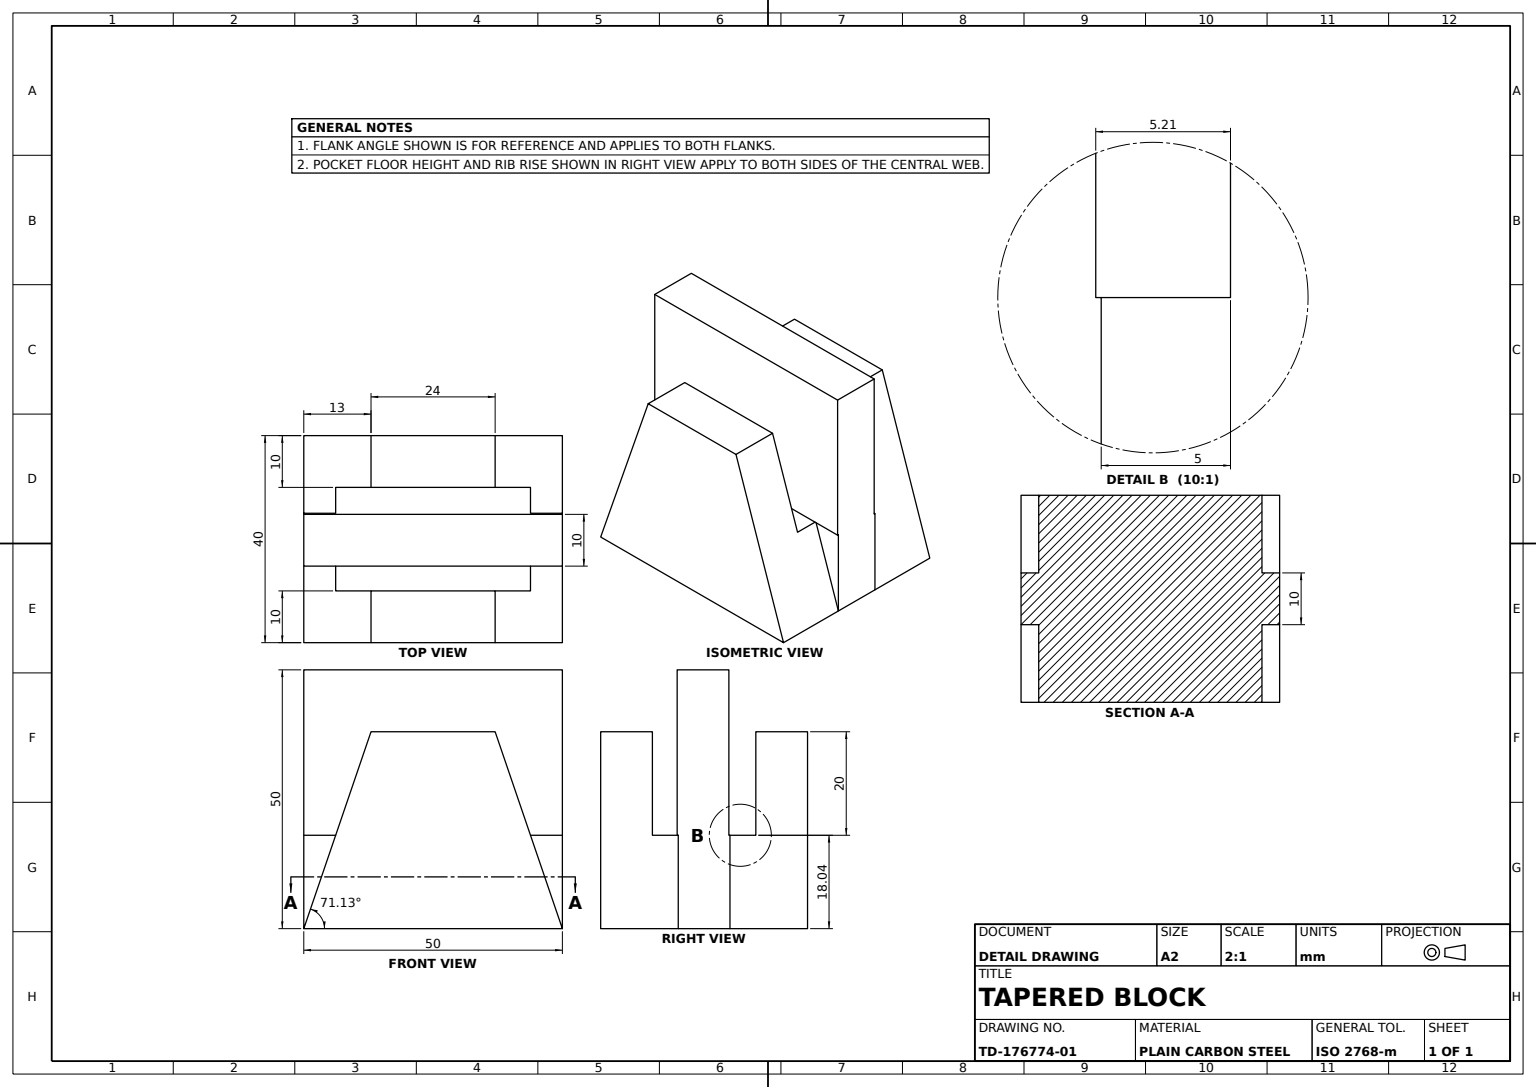
SolidWorks part; units mm, degrees
material "Plain Carbon Steel"
ref_plane "Front Plane" through (0, 0, 0) normal (0, 0, 1) x (1, 0, 0)
ref_plane "Top Plane" through (0, 0, 0) normal (0, 1, 0) x (1, 0, 0)
ref_plane "Right Plane" through (0, 0, 0) normal (1, 0, 0) x (0, 0, -1)
sketch "Base Profile Sketch" plane through (0, 0, 0) normal (0, 0, 1) x (1, 0, 0)
  line L4 (-12, 25) -> (12, 25)
  line L5 (-25, 25) -> (25, 25)
  line L6 (-25, 25) -> (-25, -25)
  line L7 (-25, -25) -> (25, -25)
  line L8 (25, 25) -> (25, -25)
  line L9 (-25, 25) -> (25, -25) construction
  line L10 (-25, -25) -> (25, 25) construction
  line L12 (-12, 13) -> (12, 13)
  line L14 (-12, 13) -> (-25, -25)
  line L15 (12, 13) -> (25, -25)
  line L16 (-25, -25) -> (25, -25)
  point P0 (0, 0)
  point P9 (0, 25)
  dimension "D1" = 50
  dimension "D2" = 50
  dimension "D3" = 24
  dimension "D4" = 12
extrude "Base Block 40mm" add sketch "Base Profile Sketch" along normal blind 40 contours L12 L15 L8 L5 L4 L6 L14 | L15 L12 L14 L7
sketch "Step Profile Cut Sketch" plane through (25, 0, 0) normal (1, 0, 0) x (0, 0, -1)
  line L0 (0, -25) -> (0, 13.0412)
  line L1 (0, 25) -> (0, -25) construction
  line L2 (0, 13.0412) -> (-10, 13.0412)
  line L3 (-10, 13.0412) -> (-10, -6.9588)
  line L4 (-10, -6.9588) -> (-15.2111, -6.9588)
  line L5 (-15.2111, -6.9588) -> (-15.2111, 25)
  line L6 (-40, 25) -> (0, 25) construction
  line L7 (-15.2111, 25) -> (-25.2111, 25)
  line L8 (-25.2111, 25) -> (-25.2111, -6.9588)
  line L9 (-25.2111, -6.9588) -> (-30, -6.9588)
  line L10 (-30, -6.9588) -> (-30, 13.0412)
  line L11 (-30, 13.0412) -> (-40, 13.0412)
  line L12 (-40, 25) -> (-40, -25) construction
  line L13 (-40, 13.0412) -> (-40, 25)
  line L14 (-40, 25) -> (-30, 25)
  line L15 (0, 13.0412) -> (0, 25)
  line L16 (0, 25) -> (-10, 25)
  line L17 (-10, 25) -> (-10, -6.9588)
  line M11 (0, -25) -> (0, 25)
  line M12 (0, 25) -> (-40, 25)
  line M13 (-40, 25) -> (-40, -25)
  dimension "D1" = 20
  dimension "D2" = 10
  dimension "D3" = 10
  dimension "D4" = 10
  dimension "D5" = 20
  dimension "D6" = 13.0412
  dimension "D7" = 5.2111
extrude "Step Profile Cut" cut sketch "Step Profile Cut Sketch" against normal through all contours L11 L10 L9 L8 M12 M13 | L17 L5 L4 L3 M12 | L17 L2 M12 M11
sketch "Pocket 24mm Sketch" plane through (0, 0, 0) normal (0, 0, -1) x (-1, 0, 0)
  line L0 (-12, 13.0412) -> (12, 13.0412)
  line L1 (25, 13.0412) -> (-25, 13.0412) construction
  line L2 (-12, 13.0412) -> (-25, -25)
  line L3 (12, 13.0412) -> (25, -25)
  line L4 (25, -25) -> (-25, -25) construction
  line L5 (25, -25) -> (25, 25)
  line L6 (25, 25) -> (-25, 25)
  line L7 (-25, 25) -> (-25, -25)
  point P5 (0, 13.0412)
  dimension "D1" = 24
  dimension "D2" = 13
extrude "Pocket 24mm x 10 Deep" cut sketch "Pocket 24mm Sketch" against normal blind 10
sketch "Pocket 12mm Sketch" plane through (0, 0, 40) normal (0, 0, 1) x (1, 0, 0)
  line L0 (-25, -25) -> (-12, 13.0412)
  line L1 (-25, 13.0412) -> (25, 13.0412) construction
  line L2 (-12, 13.0412) -> (12, 13.0412)
  line L3 (12, 13.0412) -> (25, -25)
  line L4 (25, -25) -> (25, 25)
  line L5 (25, 25) -> (-25, 25)
  line L6 (-25, 25) -> (-25, -25)
  point P10 (0, 13.0412)
  dimension "D1" = 12
  dimension "D2" = 13
extrude "Pocket 12mm x 10 Deep" cut sketch "Pocket 12mm Sketch" against normal blind 10
sketch "Triangular Cut A Sketch" plane through (0, 0, 30) normal (0, 0, 1) x (1, 0, 0)
  line L0 (-25, -25) -> (-25, -6.9588)
  line L1 (-25, -6.9588) -> (-18.8347, -6.9588)
  line L2 (-18.8347, -6.9588) -> (-25, -25)
extrude "Triangular Cut A 5mm" cut sketch "Triangular Cut A Sketch" against normal blind 5
sketch "Triangular Cut B Sketch" plane through (0, 0, 10) normal (0, 0, -1) x (-1, 0, 0)
  line L0 (25, -25) -> (25, -6.9588)
  line L1 (25, -6.9588) -> (18.8347, -6.9588)
  line L2 (12, 13.0412) -> (25, -25) construction
  line L3 (25, -6.9588) -> (-25, -6.9588) construction
  line L4 (18.8347, -6.9588) -> (25, -25)
extrude "Triangular Cut B 5mm" cut sketch "Triangular Cut B Sketch" against normal blind 5
sketch "Triangular Cut C Sketch" plane through (0, 0, 10) normal (0, 0, -1) x (-1, 0, 0)
  line L0 (-25, -25) -> (-18.8347, -6.9588)
  line L1 (-18.8347, -6.9588) -> (-25, -6.9588)
  line L2 (-25, -6.9588) -> (-25, -25)
extrude "Triangular Cut C 5mm" cut sketch "Triangular Cut C Sketch" against normal blind 5
sketch "Triangular Cut D Sketch" plane through (0, 0, 30) normal (0, 0, 1) x (1, 0, 0)
  line L0 (25, -25) -> (25, -6.9588)
  line L1 (25, -6.9588) -> (18.8347, -6.9588)
  line L2 (18.8347, -6.9588) -> (25, -25)
extrude "Triangular Cut D 5mm" cut sketch "Triangular Cut D Sketch" against normal blind 5
